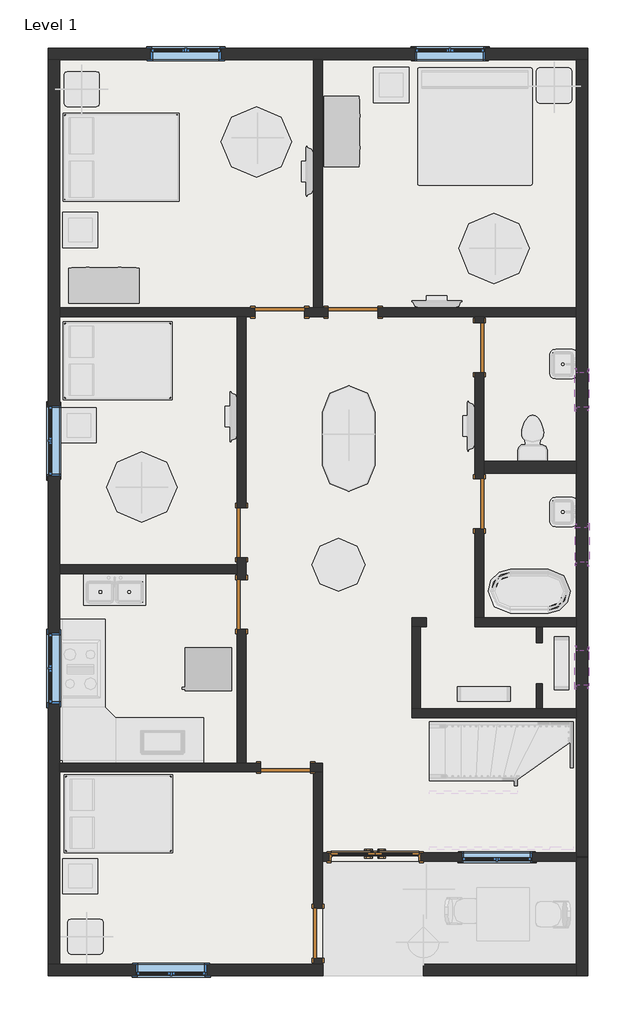
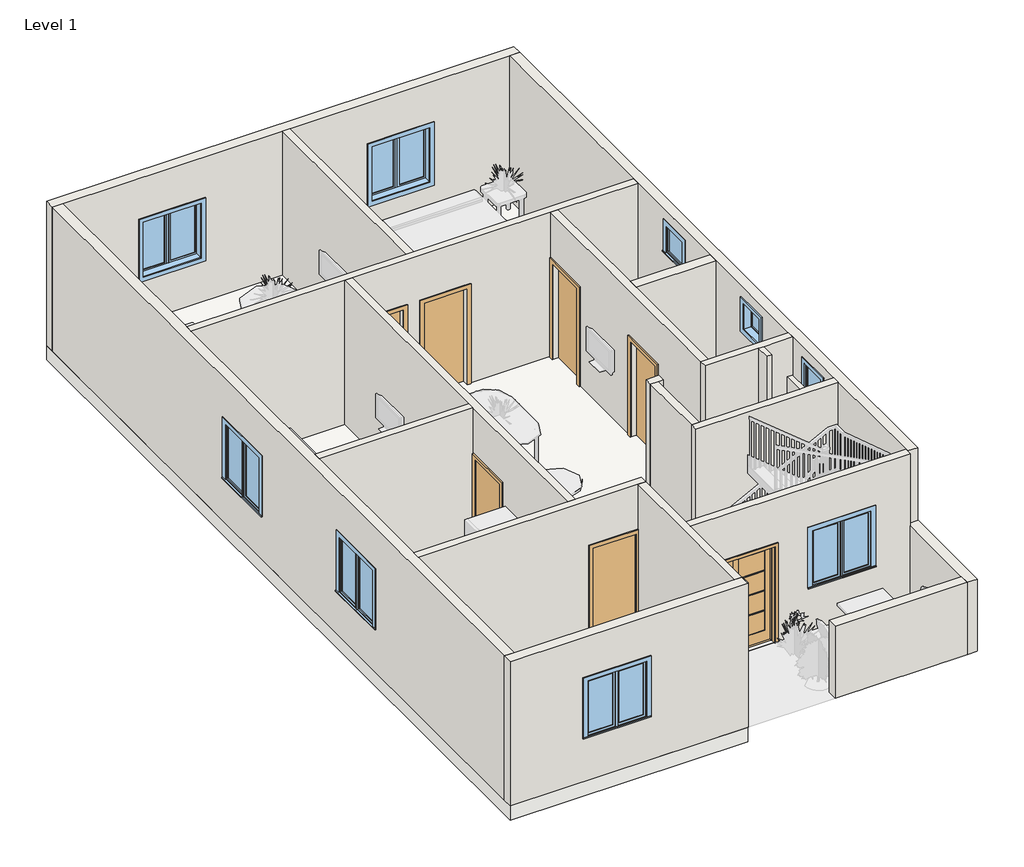
# One storey, part 1 of 3: 21 walls, 9 doors, 9 windows, 1 slab.
"""IFC4 building model written with IfcOpenShell, lengths in millimetres."""

from ifc_helpers import new_model, si_unit, frame, origin, origin_with_axes, place, context, project, spatial, polyline, outline, extrude, faceted_brep, transform, mapped, element, save
from components import door_94998e6c, door_56e8e0a9, door_706f0888, window_0862ab64, window_be30da88, window_e41d21a6

model = new_model("IFC4")

# Units and contexts
model_context = context("Model", 3, world=origin())
ifc_project = project(units=[si_unit("LENGTHUNIT", "METRE", prefix="MILLI")], contexts=[model_context])

# Site, building, storey
site = spatial("IfcSite", under=ifc_project)
building = spatial("IfcBuilding", under=site)
storey = spatial("IfcBuildingStorey", under=building, Name="Level 1", Elevation=0.0)

# Doors
placement = place(None, origin())
door_shape = door_94998e6c(model_context)
element("IfcDoor", 1, ObjectType="Door-Exterior-Double-Full Glass-Wood_Clad : 60\" x 80\"", at=placement, inside=storey, context=model_context, shape_type="MappedRepresentation", body=[
    mapped(door_shape, transform((-6580.8060487, -4568.0817046, 0.0), x_axis=(1.0, 0.0, 0.0), y_axis=(0.0, 1.0, 0.0), z_axis=(0.0, 0.0, 1.0))),
])
door_2_shape = door_56e8e0a9(model_context)
element("IfcDoor", 2, ObjectType="Single-Flush : 34\" x 80\"", at=placement, inside=storey, context=model_context, shape_type="MappedRepresentation", body=[
    mapped(door_2_shape, transform((-8231.8060487, 4852.1432954, 0.0), x_axis=(1.0, 0.0, 0.0), y_axis=(0.0, 1.0, 0.0), z_axis=(0.0, 0.0, 1.0))),
])
element("IfcDoor", 3, ObjectType="Single-Flush : 34\" x 80\"", at=placement, inside=storey, context=model_context, shape_type="MappedRepresentation", body=[
    mapped(door_2_shape, transform((-8892.2060487, -202.4567046, 0.0), x_axis=(0.0, 1.0, 0.0), y_axis=(-1.0, 0.0, 0.0), z_axis=(0.0, 0.0, 1.0))),
])
door_3_shape = door_706f0888(model_context)
element("IfcDoor", 4, ObjectType="Single-Flush : 34\" x 80\"", at=placement, inside=storey, context=model_context, shape_type="MappedRepresentation", body=[
    mapped(door_3_shape, transform((-6961.8060487, 4852.1432954, 0.0), x_axis=(-1.0, 0.0, 0.0), y_axis=(0.0, -1.0, 0.0), z_axis=(0.0, 0.0, 1.0))),
])
element("IfcDoor", 5, ObjectType="Single-Flush : 34\" x 80\"", at=placement, inside=storey, context=model_context, shape_type="MappedRepresentation", body=[
    mapped(door_3_shape, transform((-8892.2060487, 1042.1432954, 0.0), x_axis=(0.0, -1.0, 0.0), y_axis=(1.0, 0.0, 0.0), z_axis=(0.0, 0.0, 1.0))),
])
element("IfcDoor", 6, ObjectType="Single-Flush : 34\" x 80\"", at=placement, inside=storey, context=model_context, shape_type="MappedRepresentation", body=[
    mapped(door_3_shape, transform((-4777.4060487, 4242.5432954, 0.0), x_axis=(0.0, 1.0, 0.0), y_axis=(-1.0, 0.0, 0.0), z_axis=(0.0, 0.0, 1.0))),
])
element("IfcDoor", 7, ObjectType="Single-Flush : 34\" x 80\"", at=placement, inside=storey, context=model_context, shape_type="MappedRepresentation", body=[
    mapped(door_3_shape, transform((-4777.4060487, 1537.4432954, 0.0), x_axis=(0.0, 1.0, 0.0), y_axis=(-1.0, 0.0, 0.0), z_axis=(0.0, 0.0, 1.0))),
])
element("IfcDoor", 8, ObjectType="Single-Flush : 34\" x 80\"", at=placement, inside=storey, context=model_context, shape_type="MappedRepresentation", body=[
    mapped(door_3_shape, transform((-8130.2060487, -3021.8567046, 0.0), x_axis=(1.0, 0.0, 0.0), y_axis=(0.0, 1.0, 0.0), z_axis=(0.0, 0.0, 1.0))),
])
element("IfcDoor", 9, ObjectType="Single-Flush : 34\" x 80\"", at=placement, inside=storey, context=model_context, shape_type="MappedRepresentation", body=[
    mapped(door_3_shape, transform((-7571.4060487, -5892.0567046, 0.0), x_axis=(0.0, -1.0, 0.0), y_axis=(1.0, 0.0, 0.0), z_axis=(0.0, 0.0, 1.0))),
])

# Slab
element("IfcSlab", 10, ObjectType="Generic - 12\"", at=placement, inside=storey, context=model_context, shape_type="SweptSolid", body=[
    extrude(outline(polyline([(-2897.8060487, 9424.1432954), (-2897.8060487, -4583.9567046), (-2897.8060487, -4647.4567046), (-7495.2060487, -4647.4567046), (-7495.2060487, -6628.6567046), (-12245.0060487, -6628.6567046), (-12245.0060487, 9424.1432954), (-2897.8060487, 9424.1432954)])), frame((0.0, 0.0, -304.8), z_axis=(0.0, 0.0, 1.0), x_axis=(1.0, 0.0, 0.0)), (0.0, 0.0, 1.0), 304.8),
])

# Walls
element("IfcWall", 11, ObjectType="Generic - 4\"", at=placement, inside=storey, context=model_context, shape_type="SweptSolid", body=[
    extrude(outline(polyline([(-3786.8060487, -862.8567046), (-3786.8060487, -583.4567046), (-3685.2060487, -583.4567046), (-3685.2060487, -862.8567046), (-3786.8060487, -862.8567046)])), origin_with_axes(), (0.0, 0.0, 1.0), 3048.0),
])
element("IfcWall", 12, ObjectType="Generic - 4\"", at=placement, inside=storey, context=model_context, shape_type="SweptSolid", body=[
    extrude(outline(polyline([(-3786.8060487, -2005.8567046), (-3786.8060487, -1574.0567046), (-3685.2060487, -1574.0567046), (-3685.2060487, -2005.8567046), (-3786.8060487, -2005.8567046)])), origin_with_axes(), (0.0, 0.0, 1.0), 3048.0),
])
element("IfcWall", 13, ObjectType="Generic - 8\"", at=placement, inside=storey, context=model_context, shape_type="Brep", body=[
    faceted_brep([(-12245.0060487, 9220.9432954, 0.0), (-12041.8060487, 9220.9432954, 0.0), (-7647.6060487, 9220.9432954, 0.0), (-7495.2060487, 9220.9432954, 0.0), (-3101.0060487, 9220.9432954, 0.0), (-2897.8060487, 9220.9432954, 0.0), (-2897.8060487, 9220.9432954, 3048.0), (-3101.0060487, 9220.9432954, 3048.0), (-7495.2060487, 9220.9432954, 3048.0), (-7647.6060487, 9220.9432954, 3048.0), (-12041.8060487, 9220.9432954, 3048.0), (-12245.0060487, 9220.9432954, 3048.0), (-9247.8060487, 9220.9432954, 2133.6), (-9247.8060487, 9220.9432954, 914.4), (-10467.0060487, 9220.9432954, 914.4), (-10467.0060487, 9220.9432954, 2133.6), (-4675.8060487, 9220.9432954, 2133.6), (-4675.8060487, 9220.9432954, 914.4), (-5895.0060487, 9220.9432954, 914.4), (-5895.0060487, 9220.9432954, 2133.6), (-12245.0060487, 9424.1432954, 0.0), (-12245.0060487, 9424.1432954, 3048.0), (-2897.8060487, 9424.1432954, 3048.0), (-2897.8060487, 9424.1432954, 0.0), (-9247.8060487, 9424.1432954, 2133.6), (-10467.0060487, 9424.1432954, 2133.6), (-10467.0060487, 9424.1432954, 914.4), (-9247.8060487, 9424.1432954, 914.4), (-4675.8060487, 9424.1432954, 2133.6), (-5895.0060487, 9424.1432954, 2133.6), (-5895.0060487, 9424.1432954, 914.4), (-4675.8060487, 9424.1432954, 914.4)], [[[0, 1, 2, 3, 4, 5, 6, 7, 8, 9, 10, 11], [12, 13, 14, 15], [16, 17, 18, 19]], [[20, 21, 22, 23], [24, 25, 26, 27], [28, 29, 30, 31]], [[5, 4, 3, 2, 1, 0, 20, 23]], [[6, 5, 23, 22]], [[0, 11, 21, 20]], [[13, 12, 24, 27]], [[14, 13, 27, 26]], [[15, 14, 26, 25]], [[12, 15, 25, 24]], [[17, 16, 28, 31]], [[18, 17, 31, 30]], [[19, 18, 30, 29]], [[16, 19, 29, 28]], [[11, 10, 9, 8, 7, 6, 22, 21]]]),
])
element("IfcWall", 14, ObjectType="Generic - 8\"", at=placement, inside=storey, context=model_context, shape_type="Brep", body=[
    faceted_brep([(-3101.0060487, 9220.9432954, 0.0), (-3101.0060487, 4928.3432954, 0.0), (-3101.0060487, 4775.9432954, 0.0), (-3101.0060487, 2274.0432954, 0.0), (-3101.0060487, 2070.8432954, 0.0), (-3101.0060487, -431.0567046, 0.0), (-3101.0060487, -583.4567046, 0.0), (-3101.0060487, -2005.8567046, 0.0), (-3101.0060487, -2158.2567046, 0.0), (-3101.0060487, -4558.5567046, 0.0), (-3101.0060487, -4558.5567046, 3048.0), (-3101.0060487, -2158.2567046, 3048.0), (-3101.0060487, -2005.8567046, 3048.0), (-3101.0060487, -583.4567046, 3048.0), (-3101.0060487, -431.0567046, 3048.0), (-3101.0060487, 2070.8432954, 3048.0), (-3101.0060487, 2274.0432954, 3048.0), (-3101.0060487, 4775.9432954, 3048.0), (-3101.0060487, 4928.3432954, 3048.0), (-3101.0060487, 9220.9432954, 3048.0), (-3101.0060487, -989.8567046, 2768.6), (-3101.0060487, -1599.4567046, 2768.6), (-3101.0060487, -1599.4567046, 2159.0), (-3101.0060487, -989.8567046, 2159.0), (-3101.0060487, 527.7932954, 2768.6), (-3101.0060487, 527.7932954, 2159.0), (-3101.0060487, 1137.3932954, 2159.0), (-3101.0060487, 1137.3932954, 2768.6), (-3101.0060487, 3817.0932954, 2768.6), (-3101.0060487, 3207.4932954, 2768.6), (-3101.0060487, 3207.4932954, 2159.0), (-3101.0060487, 3817.0932954, 2159.0), (-2897.8060487, 9220.9432954, 0.0), (-2897.8060487, 9220.9432954, 3048.0), (-2897.8060487, -4558.5567046, 3048.0), (-2897.8060487, -4558.5567046, 0.0), (-2897.8060487, -989.8567046, 2768.6), (-2897.8060487, -989.8567046, 2159.0), (-2897.8060487, -1599.4567046, 2159.0), (-2897.8060487, -1599.4567046, 2768.6), (-2897.8060487, 527.7932954, 2768.6), (-2897.8060487, 1137.3932954, 2768.6), (-2897.8060487, 1137.3932954, 2159.0), (-2897.8060487, 527.7932954, 2159.0), (-2897.8060487, 3817.0932954, 2768.6), (-2897.8060487, 3817.0932954, 2159.0), (-2897.8060487, 3207.4932954, 2159.0), (-2897.8060487, 3207.4932954, 2768.6)], [[[0, 1, 2, 3, 4, 5, 6, 7, 8, 9, 10, 11, 12, 13, 14, 15, 16, 17, 18, 19], [20, 21, 22, 23], [24, 25, 26, 27], [28, 29, 30, 31]], [[32, 33, 34, 35], [36, 37, 38, 39], [40, 41, 42, 43], [44, 45, 46, 47]], [[9, 8, 7, 6, 5, 4, 3, 2, 1, 0, 32, 35]], [[10, 9, 35, 34]], [[0, 19, 33, 32]], [[37, 36, 20, 23]], [[38, 37, 23, 22]], [[39, 38, 22, 21]], [[36, 39, 21, 20]], [[25, 24, 40, 43]], [[26, 25, 43, 42]], [[27, 26, 42, 41]], [[24, 27, 41, 40]], [[45, 44, 28, 31]], [[46, 45, 31, 30]], [[47, 46, 30, 29]], [[44, 47, 29, 28]], [[19, 18, 17, 16, 15, 14, 13, 12, 11, 10, 34, 33]]]),
])
element("IfcWall", 15, ObjectType="Generic - 8\"", at=placement, inside=storey, context=model_context, shape_type="Brep", body=[
    faceted_brep([(-12041.8060487, -6425.4567046, 0.0), (-12041.8060487, -3098.0567046, 0.0), (-12041.8060487, -2945.6567046, 0.0), (-12041.8060487, 330.9432954, 0.0), (-12041.8060487, 483.3432954, 0.0), (-12041.8060487, 4775.9432954, 0.0), (-12041.8060487, 4928.3432954, 0.0), (-12041.8060487, 9220.9432954, 0.0), (-12041.8060487, 9220.9432954, 3048.0), (-12041.8060487, 4928.3432954, 3048.0), (-12041.8060487, 4775.9432954, 3048.0), (-12041.8060487, 483.3432954, 3048.0), (-12041.8060487, 330.9432954, 3048.0), (-12041.8060487, -2945.6567046, 3048.0), (-12041.8060487, -3098.0567046, 3048.0), (-12041.8060487, -6425.4567046, 3048.0), (-12041.8060487, -697.7567046, 2133.6), (-12041.8060487, -697.7567046, 914.4), (-12041.8060487, -1916.9567046, 914.4), (-12041.8060487, -1916.9567046, 2133.6), (-12041.8060487, 3239.2432954, 2133.6), (-12041.8060487, 3239.2432954, 914.4), (-12041.8060487, 2020.0432954, 914.4), (-12041.8060487, 2020.0432954, 2133.6), (-12245.0060487, -6425.4567046, 0.0), (-12245.0060487, -6425.4567046, 3048.0), (-12245.0060487, 9220.9432954, 3048.0), (-12245.0060487, 9220.9432954, 0.0), (-12245.0060487, -697.7567046, 2133.6), (-12245.0060487, -1916.9567046, 2133.6), (-12245.0060487, -1916.9567046, 914.4), (-12245.0060487, -697.7567046, 914.4), (-12245.0060487, 3239.2432954, 2133.6), (-12245.0060487, 2020.0432954, 2133.6), (-12245.0060487, 2020.0432954, 914.4), (-12245.0060487, 3239.2432954, 914.4)], [[[0, 1, 2, 3, 4, 5, 6, 7, 8, 9, 10, 11, 12, 13, 14, 15], [16, 17, 18, 19], [20, 21, 22, 23]], [[24, 25, 26, 27], [28, 29, 30, 31], [32, 33, 34, 35]], [[7, 6, 5, 4, 3, 2, 1, 0, 24, 27]], [[8, 7, 27, 26]], [[0, 15, 25, 24]], [[17, 16, 28, 31]], [[18, 17, 31, 30]], [[19, 18, 30, 29]], [[16, 19, 29, 28]], [[21, 20, 32, 35]], [[22, 21, 35, 34]], [[23, 22, 34, 33]], [[20, 23, 33, 32]], [[15, 14, 13, 12, 11, 10, 9, 8, 26, 25]]]),
])
element("IfcWall", 16, ObjectType="Generic - 8\"", at=placement, inside=storey, context=model_context, shape_type="SweptSolid", body=[
    extrude(outline(polyline([(-3101.0060487, 2070.8432954), (-4701.2060487, 2070.8432954), (-4701.2060487, 2274.0432954), (-3101.0060487, 2274.0432954), (-3101.0060487, 2070.8432954)])), origin_with_axes(), (0.0, 0.0, 1.0), 3048.0),
])
element("IfcWall", 17, ObjectType="Generic - 8\"", at=placement, inside=storey, context=model_context, shape_type="Brep", body=[
    faceted_brep([(-7482.5060487, -6425.4567046, 0.0), (-7495.2060487, -6425.4567046, 0.0), (-7647.6060487, -6425.4567046, 0.0), (-12041.8060487, -6425.4567046, 0.0), (-12245.0060487, -6425.4567046, 0.0), (-12245.0060487, -6425.4567046, 3048.0), (-12041.8060487, -6425.4567046, 3048.0), (-7647.6060487, -6425.4567046, 3048.0), (-7495.2060487, -6425.4567046, 3048.0), (-7482.5060487, -6425.4567046, 3048.0), (-10721.0060487, -6425.4567046, 2133.6), (-10721.0060487, -6425.4567046, 914.4), (-9501.8060487, -6425.4567046, 914.4), (-9501.8060487, -6425.4567046, 2133.6), (-7482.5060487, -6628.6567046, 0.0), (-7482.5060487, -6628.6567046, 3048.0), (-7495.2060487, -6628.6567046, 3048.0), (-12245.0060487, -6628.6567046, 3048.0), (-12245.0060487, -6628.6567046, 0.0), (-10721.0060487, -6628.6567046, 2133.6), (-9501.8060487, -6628.6567046, 2133.6), (-9501.8060487, -6628.6567046, 914.4), (-10721.0060487, -6628.6567046, 914.4)], [[[0, 1, 2, 3, 4, 5, 6, 7, 8, 9], [10, 11, 12, 13]], [[14, 15, 16, 17, 18], [19, 20, 21, 22]], [[4, 3, 2, 1, 0, 14, 18]], [[0, 9, 15, 14]], [[5, 4, 18, 17]], [[11, 10, 19, 22]], [[12, 11, 22, 21]], [[13, 12, 21, 20]], [[10, 13, 20, 19]], [[9, 8, 16, 15]], [[8, 7, 6, 5, 17, 16]]]),
])
element("IfcWall", 18, ObjectType="INNER 6\"", at=placement, inside=storey, context=model_context, shape_type="SweptSolid", body=[
    extrude(outline(polyline([(-7647.6060487, 4928.3432954), (-7647.6060487, 9220.9432954), (-7495.2060487, 9220.9432954), (-7495.2060487, 4928.3432954), (-7647.6060487, 4928.3432954)])), origin_with_axes(), (0.0, 0.0, 1.0), 3048.0),
])
element("IfcWall", 19, ObjectType="INNER 6\"", at=placement, inside=storey, context=model_context, shape_type="Brep", body=[
    faceted_brep([(-7393.6060487, 4928.3432954, 2032.0), (-7393.6060487, 4928.3432954, 0.0), (-7495.2060487, 4928.3432954, 0.0), (-7647.6060487, 4928.3432954, 0.0), (-7800.0060487, 4928.3432954, 0.0), (-7800.0060487, 4928.3432954, 2032.0), (-8663.6060487, 4928.3432954, 2032.0), (-8663.6060487, 4928.3432954, 0.0), (-12041.8060487, 4928.3432954, 0.0), (-12041.8060487, 4928.3432954, 3048.0), (-7647.6060487, 4928.3432954, 3048.0), (-7495.2060487, 4928.3432954, 3048.0), (-3101.0060487, 4928.3432954, 3048.0), (-3101.0060487, 4928.3432954, 0.0), (-6530.0060487, 4928.3432954, 0.0), (-6530.0060487, 4928.3432954, 2032.0), (-7800.0060487, 4775.9432954, 0.0), (-7393.6060487, 4775.9432954, 0.0), (-7393.6060487, 4775.9432954, 2032.0), (-6530.0060487, 4775.9432954, 2032.0), (-6530.0060487, 4775.9432954, 0.0), (-4853.6060487, 4775.9432954, 0.0), (-4701.2060487, 4775.9432954, 0.0), (-3101.0060487, 4775.9432954, 0.0), (-3101.0060487, 4775.9432954, 3048.0), (-4701.2060487, 4775.9432954, 3048.0), (-4853.6060487, 4775.9432954, 3048.0), (-8816.0060487, 4775.9432954, 3048.0), (-8968.4060487, 4775.9432954, 3048.0), (-12041.8060487, 4775.9432954, 3048.0), (-12041.8060487, 4775.9432954, 0.0), (-8968.4060487, 4775.9432954, 0.0), (-8816.0060487, 4775.9432954, 0.0), (-8663.6060487, 4775.9432954, 0.0), (-8663.6060487, 4775.9432954, 2032.0), (-7800.0060487, 4775.9432954, 2032.0)], [[[0, 1, 2, 3, 4, 5, 6, 7, 8, 9, 10, 11, 12, 13, 14, 15]], [[16, 17, 18, 19, 20, 21, 22, 23, 24, 25, 26, 27, 28, 29, 30, 31, 32, 33, 34, 35]], [[33, 32, 31, 30, 8, 7]], [[14, 13, 23, 22, 21, 20]], [[4, 3, 2, 1, 17, 16]], [[9, 8, 30, 29]], [[13, 12, 24, 23]], [[5, 4, 16, 35]], [[6, 5, 35, 34]], [[7, 6, 34, 33]], [[18, 17, 1, 0]], [[19, 18, 0, 15]], [[20, 19, 15, 14]], [[12, 11, 10, 9, 29, 28, 27, 26, 25, 24]]]),
])
element("IfcWall", 20, ObjectType="INNER 6\"", at=placement, inside=storey, context=model_context, shape_type="Brep", body=[
    faceted_brep([(-8968.4060487, 610.3432954, 0.0), (-8968.4060487, 483.3432954, 0.0), (-8968.4060487, 330.9432954, 0.0), (-8968.4060487, 229.3432954, 0.0), (-8968.4060487, 229.3432954, 2032.0), (-8968.4060487, -634.2567046, 2032.0), (-8968.4060487, -634.2567046, 0.0), (-8968.4060487, -2945.6567046, 0.0), (-8968.4060487, -2945.6567046, 3048.0), (-8968.4060487, 330.9432954, 3048.0), (-8968.4060487, 483.3432954, 3048.0), (-8968.4060487, 4775.9432954, 3048.0), (-8968.4060487, 4775.9432954, 0.0), (-8968.4060487, 1473.9432954, 0.0), (-8968.4060487, 1473.9432954, 2032.0), (-8968.4060487, 610.3432954, 2032.0), (-8816.0060487, 229.3432954, 2032.0), (-8816.0060487, 229.3432954, 0.0), (-8816.0060487, 610.3432954, 0.0), (-8816.0060487, 610.3432954, 2032.0), (-8816.0060487, 1473.9432954, 2032.0), (-8816.0060487, 1473.9432954, 0.0), (-8816.0060487, 4775.9432954, 0.0), (-8816.0060487, 4775.9432954, 3048.0), (-8816.0060487, -2945.6567046, 3048.0), (-8816.0060487, -2945.6567046, 0.0), (-8816.0060487, -634.2567046, 0.0), (-8816.0060487, -634.2567046, 2032.0)], [[[0, 1, 2, 3, 4, 5, 6, 7, 8, 9, 10, 11, 12, 13, 14, 15]], [[16, 17, 18, 19, 20, 21, 22, 23, 24, 25, 26, 27]], [[13, 12, 22, 21]], [[26, 25, 7, 6]], [[18, 17, 3, 2, 1, 0]], [[12, 11, 23, 22]], [[8, 7, 25, 24]], [[19, 18, 0, 15]], [[20, 19, 15, 14]], [[21, 20, 14, 13]], [[4, 3, 17, 16]], [[5, 4, 16, 27]], [[6, 5, 27, 26]], [[11, 10, 9, 8, 24, 23]]]),
])
element("IfcWall", 21, ObjectType="INNER 6\"", at=placement, inside=storey, context=model_context, shape_type="SweptSolid", body=[
    extrude(outline(polyline([(-12041.8060487, 483.3432954), (-8968.4060487, 483.3432954), (-8968.4060487, 330.9432954), (-12041.8060487, 330.9432954), (-12041.8060487, 483.3432954)])), origin_with_axes(), (0.0, 0.0, 1.0), 3048.0),
])
element("IfcWall", 22, ObjectType="INNER 6\"", at=placement, inside=storey, context=model_context, shape_type="Brep", body=[
    faceted_brep([(-7495.2060487, -2945.6567046, 0.0), (-7698.4060487, -2945.6567046, 0.0), (-7698.4060487, -2945.6567046, 2032.0), (-8562.0060487, -2945.6567046, 2032.0), (-8562.0060487, -2945.6567046, 0.0), (-8816.0060487, -2945.6567046, 0.0), (-8968.4060487, -2945.6567046, 0.0), (-12041.8060487, -2945.6567046, 0.0), (-12041.8060487, -2945.6567046, 3048.0), (-8968.4060487, -2945.6567046, 3048.0), (-8816.0060487, -2945.6567046, 3048.0), (-7495.2060487, -2945.6567046, 3048.0), (-7698.4060487, -3098.0567046, 2032.0), (-7698.4060487, -3098.0567046, 0.0), (-7647.6060487, -3098.0567046, 0.0), (-7495.2060487, -3098.0567046, 0.0), (-7495.2060487, -3098.0567046, 3048.0), (-7647.6060487, -3098.0567046, 3048.0), (-12041.8060487, -3098.0567046, 3048.0), (-12041.8060487, -3098.0567046, 0.0), (-8562.0060487, -3098.0567046, 0.0), (-8562.0060487, -3098.0567046, 2032.0)], [[[0, 1, 2, 3, 4, 5, 6, 7, 8, 9, 10, 11]], [[12, 13, 14, 15, 16, 17, 18, 19, 20, 21]], [[20, 19, 7, 6, 5, 4]], [[15, 14, 13, 1, 0]], [[8, 7, 19, 18]], [[0, 11, 16, 15]], [[2, 1, 13, 12]], [[3, 2, 12, 21]], [[4, 3, 21, 20]], [[11, 10, 9, 8, 18, 17, 16]]]),
])
element("IfcWall", 23, ObjectType="INNER 6\"", at=placement, inside=storey, context=model_context, shape_type="Brep", body=[
    faceted_brep([(-7495.2060487, -6425.4567046, 0.0), (-7495.2060487, -6323.8567046, 0.0), (-7495.2060487, -6323.8567046, 2032.0), (-7495.2060487, -5460.2567046, 2032.0), (-7495.2060487, -5460.2567046, 0.0), (-7495.2060487, -4647.4567046, 0.0), (-7495.2060487, -4495.0567046, 0.0), (-7495.2060487, -3098.0567046, 0.0), (-7495.2060487, -3098.0567046, 3048.0), (-7495.2060487, -4495.0567046, 3048.0), (-7495.2060487, -4647.4567046, 3048.0), (-7495.2060487, -6425.4567046, 3048.0), (-7647.6060487, -6323.8567046, 2032.0), (-7647.6060487, -6323.8567046, 0.0), (-7647.6060487, -6425.4567046, 0.0), (-7647.6060487, -6425.4567046, 3048.0), (-7647.6060487, -3098.0567046, 3048.0), (-7647.6060487, -3098.0567046, 0.0), (-7647.6060487, -5460.2567046, 0.0), (-7647.6060487, -5460.2567046, 2032.0)], [[[0, 1, 2, 3, 4, 5, 6, 7, 8, 9, 10, 11]], [[12, 13, 14, 15, 16, 17, 18, 19]], [[18, 17, 7, 6, 5, 4]], [[14, 13, 1, 0]], [[8, 7, 17, 16]], [[0, 11, 15, 14]], [[2, 1, 13, 12]], [[3, 2, 12, 19]], [[4, 3, 19, 18]], [[11, 10, 9, 8, 16, 15]]]),
])
element("IfcWall", 24, ObjectType="INNER 6\"", at=placement, inside=storey, context=model_context, shape_type="Brep", body=[
    faceted_brep([(-3101.0060487, -4647.4567046, 0.0), (-3101.0060487, -4647.4567046, 3048.0), (-7495.2060487, -4647.4567046, 3048.0), (-7495.2060487, -4647.4567046, 0.0), (-7368.2060487, -4647.4567046, 0.0), (-7368.2060487, -4647.4567046, 2057.4), (-5793.4060487, -4647.4567046, 2057.4), (-5793.4060487, -4647.4567046, 0.0), (-5082.2060487, -4647.4567046, 2133.6), (-3863.0060487, -4647.4567046, 2133.6), (-3863.0060487, -4647.4567046, 914.4), (-5082.2060487, -4647.4567046, 914.4), (-3101.0060487, -4495.0567046, 3048.0), (-3101.0060487, -4495.0567046, 0.0), (-5793.4060487, -4495.0567046, 0.0), (-5793.4060487, -4495.0567046, 2057.4), (-7368.2060487, -4495.0567046, 2057.4), (-7368.2060487, -4495.0567046, 0.0), (-7495.2060487, -4495.0567046, 0.0), (-7495.2060487, -4495.0567046, 3048.0), (-5082.2060487, -4495.0567046, 2133.6), (-5082.2060487, -4495.0567046, 914.4), (-3863.0060487, -4495.0567046, 914.4), (-3863.0060487, -4495.0567046, 2133.6), (-3101.0060487, -4583.9567046, 0.0)], [[[0, 1, 2, 3, 4, 5, 6, 7], [8, 9, 10, 11]], [[12, 13, 14, 15, 16, 17, 18, 19], [20, 21, 22, 23]], [[3, 18, 17, 4]], [[13, 24, 0, 7, 14]], [[1, 0, 24, 13, 12]], [[3, 2, 19, 18]], [[6, 15, 14, 7]], [[15, 6, 5, 16]], [[16, 5, 4, 17]], [[21, 20, 8, 11]], [[22, 21, 11, 10]], [[23, 22, 10, 9]], [[20, 23, 9, 8]], [[2, 1, 12, 19]]]),
])
element("IfcWall", 25, ObjectType="INNER 6\"", at=placement, inside=storey, context=model_context, shape_type="Brep", body=[
    faceted_brep([(-4853.6060487, 3810.7432954, 0.0), (-4853.6060487, 1969.2432954, 0.0), (-4853.6060487, 1969.2432954, 2032.0), (-4853.6060487, 1105.6432954, 2032.0), (-4853.6060487, 1105.6432954, 0.0), (-4853.6060487, -431.0567046, 0.0), (-4853.6060487, -431.0567046, 3048.0), (-4853.6060487, 4775.9432954, 3048.0), (-4853.6060487, 4775.9432954, 0.0), (-4853.6060487, 4674.3432954, 0.0), (-4853.6060487, 4674.3432954, 2032.0), (-4853.6060487, 3810.7432954, 2032.0), (-4701.2060487, 1969.2432954, 2032.0), (-4701.2060487, 1969.2432954, 0.0), (-4701.2060487, 2070.8432954, 0.0), (-4701.2060487, 2274.0432954, 0.0), (-4701.2060487, 3810.7432954, 0.0), (-4701.2060487, 3810.7432954, 2032.0), (-4701.2060487, 4674.3432954, 2032.0), (-4701.2060487, 4674.3432954, 0.0), (-4701.2060487, 4775.9432954, 0.0), (-4701.2060487, 4775.9432954, 3048.0), (-4701.2060487, 2274.0432954, 3048.0), (-4701.2060487, 2070.8432954, 3048.0), (-4701.2060487, -431.0567046, 3048.0), (-4701.2060487, -431.0567046, 0.0), (-4701.2060487, 1105.6432954, 0.0), (-4701.2060487, 1105.6432954, 2032.0)], [[[0, 1, 2, 3, 4, 5, 6, 7, 8, 9, 10, 11]], [[12, 13, 14, 15, 16, 17, 18, 19, 20, 21, 22, 23, 24, 25, 26, 27]], [[20, 19, 9, 8]], [[26, 25, 5, 4]], [[16, 15, 14, 13, 1, 0]], [[8, 7, 21, 20]], [[10, 9, 19, 18]], [[11, 10, 18, 17]], [[0, 11, 17, 16]], [[2, 1, 13, 12]], [[3, 2, 12, 27]], [[4, 3, 27, 26]], [[6, 5, 25, 24]], [[7, 6, 24, 23, 22, 21]]]),
])
element("IfcWall", 26, ObjectType="INNER 6\"", at=placement, inside=storey, context=model_context, shape_type="Brep", body=[
    faceted_brep([(-5945.8060487, -583.4567046, 0.0), (-5793.4060487, -583.4567046, 0.0), (-5691.8060487, -583.4567046, 0.0), (-5691.8060487, -583.4567046, 3048.0), (-5793.4060487, -583.4567046, 3048.0), (-5945.8060487, -583.4567046, 3048.0), (-5945.8060487, -431.0567046, 0.0), (-5945.8060487, -431.0567046, 3048.0), (-5691.8060487, -431.0567046, 3048.0), (-5691.8060487, -431.0567046, 0.0)], [[[0, 1, 2, 3, 4, 5]], [[6, 7, 8, 9]], [[2, 1, 0, 6, 9]], [[3, 2, 9, 8]], [[0, 5, 7, 6]], [[5, 4, 3, 8, 7]]]),
])
element("IfcWall", 27, ObjectType="INNER 6\"", at=placement, inside=storey, context=model_context, shape_type="Brep", body=[
    faceted_brep([(-5945.8060487, -2158.2567046, 0.0), (-3101.0060487, -2158.2567046, 0.0), (-3101.0060487, -2158.2567046, 3048.0), (-5945.8060487, -2158.2567046, 3048.0), (-5945.8060487, -2005.8567046, 0.0), (-5945.8060487, -2005.8567046, 3048.0), (-5793.4060487, -2005.8567046, 3048.0), (-3786.8060487, -2005.8567046, 3048.0), (-3685.2060487, -2005.8567046, 3048.0), (-3101.0060487, -2005.8567046, 3048.0), (-3101.0060487, -2005.8567046, 0.0), (-3685.2060487, -2005.8567046, 0.0), (-3786.8060487, -2005.8567046, 0.0), (-5793.4060487, -2005.8567046, 0.0)], [[[0, 1, 2, 3]], [[4, 5, 6, 7, 8, 9, 10, 11, 12, 13]], [[1, 0, 4, 13, 12, 11, 10]], [[2, 1, 10, 9]], [[0, 3, 5, 4]], [[3, 2, 9, 8, 7, 6, 5]]]),
])
element("IfcWall", 28, ObjectType="INNER 6\"", at=placement, inside=storey, context=model_context, shape_type="SweptSolid", body=[
    extrude(outline(polyline([(-5793.4060487, -583.4567046), (-5793.4060487, -2005.8567046), (-5945.8060487, -2005.8567046), (-5945.8060487, -583.4567046), (-5793.4060487, -583.4567046)])), origin_with_axes(), (0.0, 0.0, 1.0), 3048.0),
])
element("IfcWall", 29, ObjectType="INNER 6\"", at=placement, inside=storey, context=model_context, shape_type="Brep", body=[
    faceted_brep([(-4853.6060487, -583.4567046, 0.0), (-3786.8060487, -583.4567046, 0.0), (-3685.2060487, -583.4567046, 0.0), (-3101.0060487, -583.4567046, 0.0), (-3101.0060487, -583.4567046, 3048.0), (-3685.2060487, -583.4567046, 3048.0), (-3786.8060487, -583.4567046, 3048.0), (-4853.6060487, -583.4567046, 3048.0), (-4853.6060487, -431.0567046, 0.0), (-4853.6060487, -431.0567046, 3048.0), (-4701.2060487, -431.0567046, 3048.0), (-3101.0060487, -431.0567046, 3048.0), (-3101.0060487, -431.0567046, 0.0), (-4701.2060487, -431.0567046, 0.0)], [[[0, 1, 2, 3, 4, 5, 6, 7]], [[8, 9, 10, 11, 12, 13]], [[3, 2, 1, 0, 8, 13, 12]], [[4, 3, 12, 11]], [[0, 7, 9, 8]], [[7, 6, 5, 4, 11, 10, 9]]]),
])
element("IfcWall", 30, ObjectType="OUTER 5'", at=placement, inside=storey, context=model_context, shape_type="SweptSolid", body=[
    extrude(outline(polyline([(-5742.6060487, -6425.4567046), (-3101.0060487, -6425.4567046), (-3101.0060487, -6628.6567046), (-5742.6060487, -6628.6567046), (-5742.6060487, -6425.4567046)])), origin_with_axes(), (0.0, 0.0, 1.0), 1524.0),
])
element("IfcWall", 31, ObjectType="OUTER 5'", at=placement, inside=storey, context=model_context, shape_type="Brep", body=[
    faceted_brep([(-3101.0060487, -4583.9567046, 0.0), (-3101.0060487, -4647.4567046, 0.0), (-3101.0060487, -6425.4567046, 0.0), (-3101.0060487, -6628.6567046, 0.0), (-3101.0060487, -6628.6567046, 1524.0), (-3101.0060487, -6425.4567046, 1524.0), (-3101.0060487, -4583.9567046, 1524.0), (-2897.8060487, -4583.9567046, 0.0), (-2897.8060487, -4583.9567046, 1524.0), (-2897.8060487, -6628.6567046, 1524.0), (-2897.8060487, -6628.6567046, 0.0)], [[[0, 1, 2, 3, 4, 5, 6]], [[7, 8, 9, 10]], [[3, 2, 1, 0, 7, 10]], [[6, 5, 4, 9, 8]], [[0, 6, 8, 7]], [[4, 3, 10, 9]]]),
])

# Windows
window_shape = window_0862ab64(model_context)
element("IfcWindow", 32, ObjectType="Casement Dbl with Trim : 48\" x 48\"", at=placement, inside=storey, context=model_context, shape_type="MappedRepresentation", body=[
    mapped(window_shape, transform((-9857.4060487, 9303.4932954, 0.0), x_axis=(1.0, 0.0, 0.0), y_axis=(0.0, 1.0, 0.0), z_axis=(0.0, 0.0, 1.0))),
])
element("IfcWindow", 33, ObjectType="Casement Dbl with Trim : 48\" x 48\"", at=placement, inside=storey, context=model_context, shape_type="MappedRepresentation", body=[
    mapped(window_shape, transform((-5285.4060487, 9303.4932954, 0.0), x_axis=(1.0, 0.0, 0.0), y_axis=(0.0, 1.0, 0.0), z_axis=(0.0, 0.0, 1.0))),
])
element("IfcWindow", 34, ObjectType="Casement Dbl with Trim : 48\" x 48\"", at=placement, inside=storey, context=model_context, shape_type="MappedRepresentation", body=[
    mapped(window_shape, transform((-10111.4060487, -6508.0067046, 0.0), x_axis=(-1.0, 0.0, 0.0), y_axis=(0.0, -1.0, 0.0), z_axis=(0.0, 0.0, 1.0))),
])
element("IfcWindow", 35, ObjectType="Casement Dbl with Trim : 48\" x 48\"", at=placement, inside=storey, context=model_context, shape_type="MappedRepresentation", body=[
    mapped(window_shape, transform((-12124.3560487, -1307.3567046, 0.0), x_axis=(0.0, 1.0, 0.0), y_axis=(-1.0, 0.0, 0.0), z_axis=(0.0, 0.0, 1.0))),
])
element("IfcWindow", 36, ObjectType="Casement Dbl with Trim : 48\" x 48\"", at=placement, inside=storey, context=model_context, shape_type="MappedRepresentation", body=[
    mapped(window_shape, transform((-12124.3560487, 2629.6432954, 0.0), x_axis=(0.0, 1.0, 0.0), y_axis=(-1.0, 0.0, 0.0), z_axis=(0.0, 0.0, 1.0))),
])
window_2_shape = window_be30da88(model_context)
element("IfcWindow", 37, ObjectType="Casement Dbl with Trim : 48\" x 48\"", at=placement, inside=storey, context=model_context, shape_type="MappedRepresentation", body=[
    mapped(window_2_shape, transform((-4472.6060487, -4552.2067046, 0.0), x_axis=(-1.0, 0.0, 0.0), y_axis=(0.0, -1.0, 0.0), z_axis=(0.0, 0.0, 1.0))),
])
window_3_shape = window_e41d21a6(model_context)
element("IfcWindow", 38, ObjectType="Transom with Trim : 24\" x 24\"", at=placement, inside=storey, context=model_context, shape_type="MappedRepresentation", body=[
    mapped(window_3_shape, transform((-2999.4060487, -1256.5567046, 0.0), x_axis=(0.0, 1.0, 0.0), y_axis=(-1.0, 0.0, 0.0), z_axis=(0.0, 0.0, 1.0))),
])
element("IfcWindow", 39, ObjectType="Transom with Trim : 24\" x 24\"", at=placement, inside=storey, context=model_context, shape_type="MappedRepresentation", body=[
    mapped(window_3_shape, transform((-2999.4060487, 794.4932954, 0.0), x_axis=(0.0, -1.0, 0.0), y_axis=(1.0, 0.0, 0.0), z_axis=(0.0, 0.0, 1.0))),
])
element("IfcWindow", 40, ObjectType="Transom with Trim : 24\" x 24\"", at=placement, inside=storey, context=model_context, shape_type="MappedRepresentation", body=[
    mapped(window_3_shape, transform((-2999.4060487, 3550.3932954, 0.0), x_axis=(0.0, 1.0, 0.0), y_axis=(-1.0, 0.0, 0.0), z_axis=(0.0, 0.0, 1.0))),
])

save(model, "model.ifc")

# Revit data of these elements
# Type "Door-Exterior-Double-Full Glass-Wood_Clad : 60\" x 80\""
#   Type Mark = "8"
#   Assembly Code = "B2030100"
#   Analytic Construction = "French door, wood frame with double glass"
#   Top Rail = 0' - 4 11/16"
#   Threshold Offset [instance default] = 0' - 0 1/2"
#   Thickness = 0' - 1 3/8"
#   Thermal Resistance (R) = 1.9158 (h·ft²·°F)/BTU
#   Swing Angle [instance default] = 90.00°
#   Stiles = 0' - 4 3/4"
#   Rough Width = 5' - 2"
#   Rough Height = 6' - 9"
#   Panel Width = 2' - 6"
#   Door Offset [instance default] = 0' - 0"
#   Height = 6' - 8"
#   Width = 5' - 0"
#   Heat Transfer Coefficient (U) = 0.5220 BTU/(h·ft²·°F)
#   Bottom Rail = 0' - 9 1/8"
#   Exterior Trim [instance default] = yes
#   Threshold [instance default] = yes
#   Show Grill [instance default] = yes
#   Function = 1
#   Trim Material = Cherry
#   Threshold Material = Cherry
#   Panel Material = Cherry
#   Glazing = Glass
#   Frame Material = Cherry
#   Door Handle Material = Aluminum
#   Visual Light Transmittance = 0
#   Solar Heat Gain Coefficient = 0
#   Wall Closure = (empty or 0)
#   Construction Type = (empty or 0)
# Type "Single-Flush : 34\" x 80\""
#   Type Mark = "7"
#   Construction Type Id = "MDOOR"
#   Assembly Code = "C1020"
#   Analytic Construction = "Metal"
#   Thickness = 0' - 2"
#   Heat Transfer Coefficient (U) = 0.651978 BTU/(h·ft²·°F)
#   Height = 6' - 8"
#   Trim Projection Ext = 0' - 1"
#   Trim Projection Int = 0' - 1"
#   Trim Width = 0' - 3"
#   Width = 2' - 10"
#   Define Thermal Properties by = 1
#   Door Material = Door - Panel
#   Frame Material = Door - Frame
#   Visual Light Transmittance = 0
#   Solar Heat Gain Coefficient = 0
#   Function = (empty or 0)
#   Wall Closure = (empty or 0)
# Type "Generic - 12\""
#   Assembly Code = "B1010"
#   Function = 0
#   Layers, outside or top first: 1' - 0" no material (function 1)
# Type "Generic - 4\""
#   Assembly Code = "B2010"
#   Layers, outside or top first: 0' - 4" "Brick, Common" (function 1)
# Type "Generic - 8\""
#   Assembly Code = "B2010"
#   Layers, outside or top first: 0' - 8" "Brick, Common" (function 1)
# Type "INNER 6\""
#   Assembly Code = "B2010"
#   Layers, outside or top first: 0' - 6" "Brick, Common" (function 1)
# Type "OUTER 5'"
#   Assembly Code = "B2010"
#   Layers, outside or top first: 0' - 8" "Birch" (function 1)
# Type "Casement Dbl with Trim : 48\" x 48\""
#   Type Mark = "10"
#   Construction Type Id = "GSP4R"
#   Assembly Code = "B2020100"
#   Analytic Construction = "1/8 in Pilkington single glazing"
#   Visual Light Transmittance = 0.9
#   Solar Heat Gain Coefficient = 0.78
#   Heat Transfer Coefficient (U) = 0.6496 BTU/(h·ft²·°F)
#   Height = 4' - 0"
#   Default Sill Height = 3' - 0"
#   Trim Projection - Ext. = 0' - 0 1/2"
#   Trim Projection - Int. = 0' - 0 3/4"
#   Trim Width - Exterior = 0' - 3 1/2"
#   Trim Width - Interior = 0' - 3 1/2"
#   Width = 4' - 0"
#   Window Inset = 0' - 0 3/4"
#   Define Thermal Properties by = 1
#   Glass Pane Material = Glass
#   Sash Material = Sash
#   Trim Exterior Material = Trim
#   Trim Interior Material = Trim
#   Wall Closure = (empty or 0)
# Type "Transom with Trim : 24\" x 24\""
#   Type Mark = "13"
#   Construction Type Id = "GSP4R"
#   Assembly Code = "B2020100"
#   Analytic Construction = "1/8 in Pilkington single glazing"
#   Visual Light Transmittance = 0.9
#   Solar Heat Gain Coefficient = 0.78
#   Heat Transfer Coefficient (U) = 0.6496 BTU/(h·ft²·°F)
#   Height = 2' - 0"
#   Default Sill Height = 7' - 1"
#   Trim Projection - Ext. = 0' - 0 1/2"
#   Trim Projection - Int. = 0' - 0 3/4"
#   Trim Width - Exterior = 0' - 3 1/2"
#   Trim Width - Interior = 0' - 3 1/2"
#   Width = 2' - 0"
#   Window Inset = 0' - 0 3/4"
#   Define Thermal Properties by = 1
#   Glass Pane Material = Glass
#   Sash Material = Sash
#   Trim Exterior Material = Trim
#   Trim Interior Material = Trim
#   Wall Closure = (empty or 0)
# Element 1 (IfcDoor, "Door-Exterior-Double-Full Glass-Wood_Clad : 60\" x 80\"")
#   Threshold Offset = 0' - 0 1/2"
#   Swing Angle = 90.00°
#   Door Offset = 0' - 0"
#   Threshold = yes
#   Show Grill = yes
#   Exterior Trim = yes
#   Phase Created = New Construction
#   Materials on its faces: "Cherry", "Aluminum", "Glass"
# Elements 2, 3, 4, 5, 6, 7, 8, 9 (IfcDoor, "Single-Flush : 34\" x 80\"")
#   Phase Created = New Construction
#   Materials on its faces: "Door - Frame", "Door - Panel"
# Element 10 (IfcSlab, "Generic - 12\"")
#   Height Offset From Level = 0' - 0"
#   Phase Created = New Construction
#   Materials on its faces: "Default Floor"
# Elements 11, 12 (IfcWall, "Generic - 4\"")
#   Top Offset = 0' - 0"
#   Base Offset = 0' - 0"
#   Unconnected Height = 10' - 0"
#   wall height = 10' - 0"
#   Phase Created = New Construction
#   Base Constraint = Level 1
#   Materials on its faces: "Brick, Common"
# Elements 13, 14, 15, 16, 17 (IfcWall, "Generic - 8\"")
#   Top Offset = 0' - 0"
#   Base Offset = 0' - 0"
#   Unconnected Height = 10' - 0"
#   wall height = 10' - 0"
#   Phase Created = New Construction
#   Base Constraint = Level 1
#   Materials on its faces: "Brick, Common"
# Elements 18, 19, 20, 21, 22, 23, 24, 25, 26, 27, 28, 29 (IfcWall, "INNER 6\"")
#   Top Offset = 0' - 0"
#   Base Offset = 0' - 0"
#   Unconnected Height = 10' - 0"
#   wall height = 10' - 0"
#   Phase Created = New Construction
#   Base Constraint = Level 1
#   Materials on its faces: "Brick, Common"
# Elements 30, 31 (IfcWall, "OUTER 5'")
#   Top Offset = 0' - 0"
#   Base Offset = 0' - 0"
#   Unconnected Height = 5' - 0"
#   wall height = 5' - 0"
#   Phase Created = New Construction
#   Base Constraint = Level 1
#   Materials on its faces: "Birch"
# Element 32 (IfcWindow, "Casement Dbl with Trim : 48\" x 48\"")
#   Mark = "1"
#   Phase Created = New Construction
#   Materials on its faces: "Sash", "Trim", "Glass"
# Element 33 (IfcWindow, "Casement Dbl with Trim : 48\" x 48\"")
#   Mark = "2"
#   Phase Created = New Construction
#   Materials on its faces: "Sash", "Trim", "Glass"
# Element 34 (IfcWindow, "Casement Dbl with Trim : 48\" x 48\"")
#   Mark = "3"
#   Phase Created = New Construction
#   Materials on its faces: "Sash", "Trim", "Glass"
# Element 35 (IfcWindow, "Casement Dbl with Trim : 48\" x 48\"")
#   Mark = "5"
#   Phase Created = New Construction
#   Materials on its faces: "Sash", "Trim", "Glass"
# Element 36 (IfcWindow, "Casement Dbl with Trim : 48\" x 48\"")
#   Mark = "6"
#   Phase Created = New Construction
#   Materials on its faces: "Sash", "Trim", "Glass"
# Element 37 (IfcWindow, "Casement Dbl with Trim : 48\" x 48\"")
#   Mark = "4"
#   Phase Created = New Construction
#   Materials on its faces: "Sash", "Trim", "Glass"
# Element 38 (IfcWindow, "Transom with Trim : 24\" x 24\"")
#   Mark = "7"
#   Phase Created = New Construction
#   Materials on its faces: "Sash", "Trim", "Glass"
# Element 39 (IfcWindow, "Transom with Trim : 24\" x 24\"")
#   Mark = "8"
#   Phase Created = New Construction
#   Materials on its faces: "Sash", "Trim", "Glass"
# Element 40 (IfcWindow, "Transom with Trim : 24\" x 24\"")
#   Mark = "9"
#   Phase Created = New Construction
#   Materials on its faces: "Sash", "Trim", "Glass"
# Materials
#   "Cherry": class "Wood", colour RGB 226 177 128, transparency 0, Description = "Prunus Serotina", Cost = 0
#   "Glass": class "Glass", colour RGB 0 128 192, transparency 0.75, Description = "Soda Lime Glass", Cost = 0
#   "Aluminum": class "Metal", colour RGB 247 247 247, transparency 0, Description = "Aluminum 6061", Cost = 0
#   "Door - Panel": class "Wood", colour RGB 210 159 95, transparency 0
#   "Door - Frame": colour RGB 118 70 51, transparency 0
#   "Brick, Common": class "Masonry", colour RGB 170 98 104, transparency 0, Description = "Common brick", Cost = 0
#   "Birch": class "Wood", colour RGB 224 178 126, transparency 0, Description = "Betula Alleghaniensis", Cost = 0
#   "Sash": class "Wood", colour RGB 224 178 126, transparency 0
#   "Trim": class "Wood", colour RGB 224 178 126, transparency 0
#   "Default Floor": colour RGB 128 128 128, transparency 0
# Room at (-9908.926, 7045.421) mm, phase "New Construction", upper level "Level 1", upper offset 10' - 0", lower offset 0' - 0"
#   Number = "1"
#   Name = "BEDROOM"
# Room at (-5466.911, 6912.687) mm, phase "New Construction", upper level "Level 1", upper offset 10' - 0", lower offset 0' - 0"
#   Number = "2"
#   Name = "BEDROOM"
# Room at (-10401.675, 2504.045) mm, phase "New Construction", upper level "Level 1", upper offset 10' - 0", lower offset 0' - 0"
#   Number = "3"
#   Name = "BEDROOM"
# Room at (-3842.864, 3002.325) mm, phase "New Construction", upper level "Level 1", upper offset 10' - 0", lower offset 0' - 0"
#   Number = "4"
#   Name = "TOILET"
# Room at (-3842.864, 615.423) mm, phase "New Construction", upper level "Level 1", upper offset 10' - 0", lower offset 0' - 0"
#   Number = "5"
#   Name = "BATH"
# Room at (-6800.277, 1740.17) mm, phase "New Construction", upper level "Level 1", upper offset 10' - 0", lower offset 0' - 0"
#   Number = "6"
#   Name = "LIVING/DINING HALL"
# Room at (-10578.187, -1750.134) mm, phase "New Construction", upper level "Level 1", upper offset 10' - 0", lower offset 0' - 0"
#   Number = "7"
#   Name = "KITCHEN"
# Room at (-9788.18, -5221.754) mm, phase "New Construction", upper level "Level 1", upper offset 10' - 0", lower offset 0' - 0"
#   Number = "8"
#   Name = "GUEST ROOM"
# Room at (-4577.309, -1548.011) mm, phase "New Construction", upper level "Level 1", upper offset 10' - 0", lower offset 0' - 0"
#   Number = "9"
# Room at (-5002.205, -5751.203) mm, phase "New Construction", upper level "Level 1", upper offset 10' - 0", lower offset 0' - 0"
#   Number = "10"
